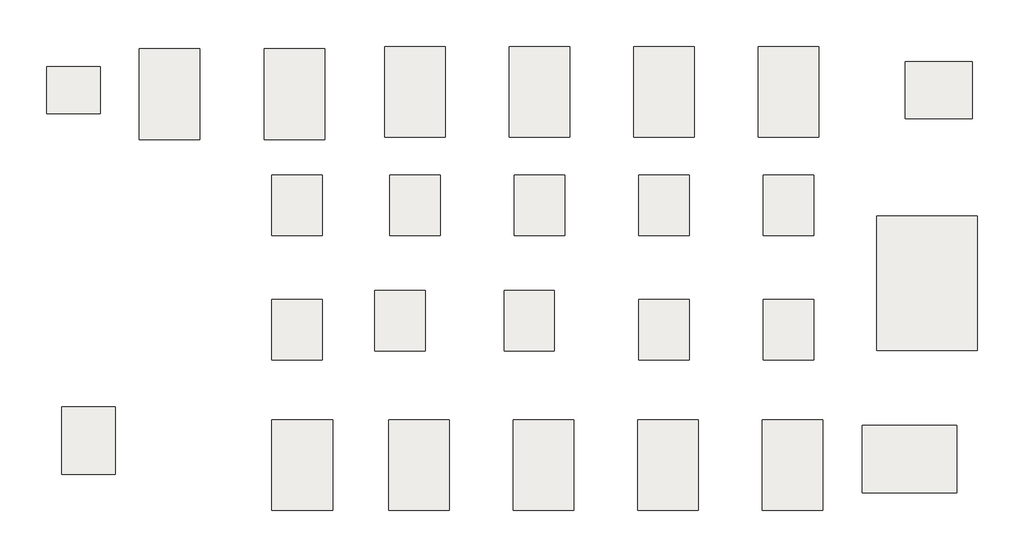
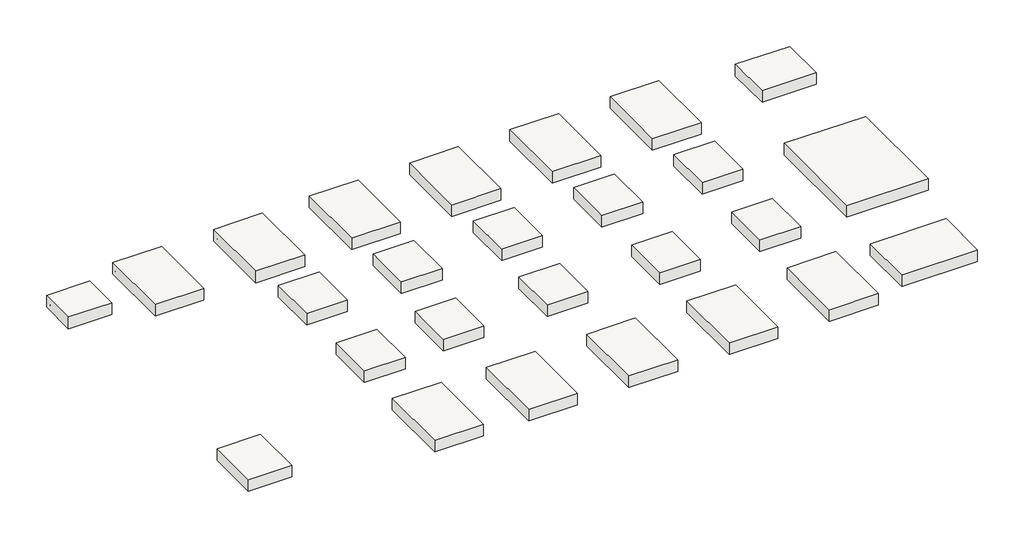
# One storey, part 1 of 2: 26 slabs.
"""IFC4 building model written with IfcOpenShell, lengths in millimetres."""

from ifc_helpers import new_model, si_unit, origin, place, context, project, spatial, transform, mapped, element, save
from components import m_footing_rectangular_1500_x_1800_x_450mm_b88d8e73, m_footing_rectangular_1600_x_1400_x_450mm_70e385b2, m_footing_rectangular_1600_x_2000_x_450mm_9aacb398, m_footing_rectangular_1800_x_2700_x_450mm_20c57781, m_footing_rectangular_2000_x_1700_x_450mm_1621679d, m_footing_rectangular_2800_x_2000_x_450mm_3d0566a5, m_footing_rectangular_3000_x_4000_x_450mm_fa7846ad

model = new_model("IFC4")

# Units and contexts
model_context = context("Model", 3, world=origin())
ifc_project = project(units=[si_unit("LENGTHUNIT", "METRE", prefix="MILLI")], contexts=[model_context])

# Site, building, storey
site = spatial("IfcSite", under=ifc_project)
building = spatial("IfcBuilding", under=site)
storey = spatial("IfcBuildingStorey", under=building, Elevation=-2133.6)

# Slabs
placement = place(None, origin())
m_footing_rectangular_1500_x_1800_x_450mm_shape = m_footing_rectangular_1500_x_1800_x_450mm_b88d8e73(model_context)
element("IfcSlab", 1, ObjectType="M_Footing-Rectangular : 1500 x 1800 x 450mm", at=placement, inside=storey, context=model_context, shape_type="MappedRepresentation", body=[
    mapped(m_footing_rectangular_1500_x_1800_x_450mm_shape, transform((-8871.6002151, 1284.1968026, -2133.6), x_axis=(1.0, 0.0, 0.0), y_axis=(0.0, 1.0, 0.0), z_axis=(0.0, 0.0, 1.0))),
])
element("IfcSlab", 2, ObjectType="M_Footing-Rectangular : 1500 x 1800 x 450mm", at=placement, inside=storey, context=model_context, shape_type="MappedRepresentation", body=[
    mapped(m_footing_rectangular_1500_x_1800_x_450mm_shape, transform((-5370.5486955, 1285.6388796, -2133.6), x_axis=(1.0, 0.0, 0.0), y_axis=(0.0, 1.0, 0.0), z_axis=(0.0, 0.0, 1.0))),
])
element("IfcSlab", 3, ObjectType="M_Footing-Rectangular : 1500 x 1800 x 450mm", at=placement, inside=storey, context=model_context, shape_type="MappedRepresentation", body=[
    mapped(m_footing_rectangular_1500_x_1800_x_450mm_shape, transform((2029.4513045, 1285.6388796, -2133.6), x_axis=(1.0, 0.0, 0.0), y_axis=(0.0, 1.0, 0.0), z_axis=(0.0, 0.0, 1.0))),
])
element("IfcSlab", 4, ObjectType="M_Footing-Rectangular : 1500 x 1800 x 450mm", at=placement, inside=storey, context=model_context, shape_type="MappedRepresentation", body=[
    mapped(m_footing_rectangular_1500_x_1800_x_450mm_shape, transform((5729.4513045, 1285.6388796, -2133.6), x_axis=(1.0, 0.0, 0.0), y_axis=(0.0, 1.0, 0.0), z_axis=(0.0, 0.0, 1.0))),
])
element("IfcSlab", 5, ObjectType="M_Footing-Rectangular : 1500 x 1800 x 450mm", at=placement, inside=storey, context=model_context, shape_type="MappedRepresentation", body=[
    mapped(m_footing_rectangular_1500_x_1800_x_450mm_shape, transform((-8870.5486955, -2415.8031974, -2133.6), x_axis=(1.0, 0.0, 0.0), y_axis=(0.0, 1.0, 0.0), z_axis=(0.0, 0.0, 1.0))),
])
element("IfcSlab", 6, ObjectType="M_Footing-Rectangular : 1500 x 1800 x 450mm", at=placement, inside=storey, context=model_context, shape_type="MappedRepresentation", body=[
    mapped(m_footing_rectangular_1500_x_1800_x_450mm_shape, transform((-5810.4090662, -2148.9247482, -2133.6), x_axis=(1.0, 0.0, 0.0), y_axis=(0.0, 1.0, 0.0), z_axis=(0.0, 0.0, 1.0))),
])
element("IfcSlab", 7, ObjectType="M_Footing-Rectangular : 1500 x 1800 x 450mm", at=placement, inside=storey, context=model_context, shape_type="MappedRepresentation", body=[
    mapped(m_footing_rectangular_1500_x_1800_x_450mm_shape, transform((-1974.31456, -2148.9247482, -2133.6), x_axis=(1.0, 0.0, 0.0), y_axis=(0.0, 1.0, 0.0), z_axis=(0.0, 0.0, 1.0))),
])
element("IfcSlab", 8, ObjectType="M_Footing-Rectangular : 1500 x 1800 x 450mm", at=placement, inside=storey, context=model_context, shape_type="MappedRepresentation", body=[
    mapped(m_footing_rectangular_1500_x_1800_x_450mm_shape, transform((2029.4513045, -2415.8031974, -2133.6), x_axis=(1.0, 0.0, 0.0), y_axis=(0.0, 1.0, 0.0), z_axis=(0.0, 0.0, 1.0))),
])
element("IfcSlab", 9, ObjectType="M_Footing-Rectangular : 1500 x 1800 x 450mm", at=placement, inside=storey, context=model_context, shape_type="MappedRepresentation", body=[
    mapped(m_footing_rectangular_1500_x_1800_x_450mm_shape, transform((5729.4513045, -2415.8031974, -2133.6), x_axis=(1.0, 0.0, 0.0), y_axis=(0.0, 1.0, 0.0), z_axis=(0.0, 0.0, 1.0))),
])
element("IfcSlab", 10, ObjectType="M_Footing-Rectangular : 1500 x 1800 x 450mm", at=placement, inside=storey, context=model_context, shape_type="MappedRepresentation", body=[
    mapped(m_footing_rectangular_1500_x_1800_x_450mm_shape, transform((-1670.5486955, 1285.6388796, -2133.6), x_axis=(1.0, 0.0, 0.0), y_axis=(0.0, 1.0, 0.0), z_axis=(0.0, 0.0, 1.0))),
])
m_footing_rectangular_1600_x_1400_x_450mm_shape = m_footing_rectangular_1600_x_1400_x_450mm_70e385b2(model_context)
element("IfcSlab", 11, ObjectType="M_Footing-Rectangular : 1600 x 1400 x 450mm", at=placement, inside=storey, context=model_context, shape_type="MappedRepresentation", body=[
    mapped(m_footing_rectangular_1600_x_1400_x_450mm_shape, transform((-15520.5877753, 4707.7547256, -2133.6), x_axis=(1.0, 0.0, 0.0), y_axis=(0.0, 1.0, 0.0), z_axis=(0.0, 0.0, 1.0))),
])
m_footing_rectangular_1600_x_2000_x_450mm_shape = m_footing_rectangular_1600_x_2000_x_450mm_9aacb398(model_context)
element("IfcSlab", 12, ObjectType="M_Footing-Rectangular : 1600 x 2000 x 450mm", at=placement, inside=storey, context=model_context, shape_type="MappedRepresentation", body=[
    mapped(m_footing_rectangular_1600_x_2000_x_450mm_shape, transform((-15072.8289366, -5717.2452744, -2133.6), x_axis=(1.0, 0.0, 0.0), y_axis=(0.0, 1.0, 0.0), z_axis=(0.0, 0.0, 1.0))),
])
m_footing_rectangular_1800_x_2700_x_450mm_shape = m_footing_rectangular_1800_x_2700_x_450mm_20c57781(model_context)
element("IfcSlab", 13, ObjectType="M_Footing-Rectangular : 1800 x 2700 x 450mm", at=placement, inside=storey, context=model_context, shape_type="MappedRepresentation", body=[
    mapped(m_footing_rectangular_1800_x_2700_x_450mm_shape, transform((-12666.802732, 4582.7547256, -2133.6), x_axis=(1.0, 0.0, 0.0), y_axis=(0.0, 1.0, 0.0), z_axis=(0.0, 0.0, 1.0))),
])
element("IfcSlab", 14, ObjectType="M_Footing-Rectangular : 1800 x 2700 x 450mm", at=placement, inside=storey, context=model_context, shape_type="MappedRepresentation", body=[
    mapped(m_footing_rectangular_1800_x_2700_x_450mm_shape, transform((-8950.302732, 4582.7547256, -2133.6), x_axis=(1.0, 0.0, 0.0), y_axis=(0.0, 1.0, 0.0), z_axis=(0.0, 0.0, 1.0))),
])
element("IfcSlab", 15, ObjectType="M_Footing-Rectangular : 1800 x 2700 x 450mm", at=placement, inside=storey, context=model_context, shape_type="MappedRepresentation", body=[
    mapped(m_footing_rectangular_1800_x_2700_x_450mm_shape, transform((-5375.302732, 4654.6486596, -2133.6), x_axis=(1.0, 0.0, 0.0), y_axis=(0.0, 1.0, 0.0), z_axis=(0.0, 0.0, 1.0))),
])
element("IfcSlab", 16, ObjectType="M_Footing-Rectangular : 1800 x 2700 x 450mm", at=placement, inside=storey, context=model_context, shape_type="MappedRepresentation", body=[
    mapped(m_footing_rectangular_1800_x_2700_x_450mm_shape, transform((-1675.302732, 4654.6486596, -2133.6), x_axis=(1.0, 0.0, 0.0), y_axis=(0.0, 1.0, 0.0), z_axis=(0.0, 0.0, 1.0))),
])
element("IfcSlab", 17, ObjectType="M_Footing-Rectangular : 1800 x 2700 x 450mm", at=placement, inside=storey, context=model_context, shape_type="MappedRepresentation", body=[
    mapped(m_footing_rectangular_1800_x_2700_x_450mm_shape, transform((2024.697268, 4654.6486596, -2133.6), x_axis=(1.0, 0.0, 0.0), y_axis=(0.0, 1.0, 0.0), z_axis=(0.0, 0.0, 1.0))),
])
element("IfcSlab", 18, ObjectType="M_Footing-Rectangular : 1800 x 2700 x 450mm", at=placement, inside=storey, context=model_context, shape_type="MappedRepresentation", body=[
    mapped(m_footing_rectangular_1800_x_2700_x_450mm_shape, transform((5724.697268, 4654.6486596, -2133.6), x_axis=(1.0, 0.0, 0.0), y_axis=(0.0, 1.0, 0.0), z_axis=(0.0, 0.0, 1.0))),
])
element("IfcSlab", 19, ObjectType="M_Footing-Rectangular : 1800 x 2700 x 450mm", at=placement, inside=storey, context=model_context, shape_type="MappedRepresentation", body=[
    mapped(m_footing_rectangular_1800_x_2700_x_450mm_shape, transform((-8720.5486955, -6446.5229254, -2133.6), x_axis=(1.0, 0.0, 0.0), y_axis=(0.0, 1.0, 0.0), z_axis=(0.0, 0.0, 1.0))),
])
element("IfcSlab", 20, ObjectType="M_Footing-Rectangular : 1800 x 2700 x 450mm", at=placement, inside=storey, context=model_context, shape_type="MappedRepresentation", body=[
    mapped(m_footing_rectangular_1800_x_2700_x_450mm_shape, transform((-5250.302732, -6446.5229254, -2133.6), x_axis=(1.0, 0.0, 0.0), y_axis=(0.0, 1.0, 0.0), z_axis=(0.0, 0.0, 1.0))),
])
element("IfcSlab", 21, ObjectType="M_Footing-Rectangular : 1800 x 2700 x 450mm", at=placement, inside=storey, context=model_context, shape_type="MappedRepresentation", body=[
    mapped(m_footing_rectangular_1800_x_2700_x_450mm_shape, transform((-1550.302732, -6446.5229254, -2133.6), x_axis=(1.0, 0.0, 0.0), y_axis=(0.0, 1.0, 0.0), z_axis=(0.0, 0.0, 1.0))),
])
element("IfcSlab", 22, ObjectType="M_Footing-Rectangular : 1800 x 2700 x 450mm", at=placement, inside=storey, context=model_context, shape_type="MappedRepresentation", body=[
    mapped(m_footing_rectangular_1800_x_2700_x_450mm_shape, transform((2149.697268, -6446.5229254, -2133.6), x_axis=(1.0, 0.0, 0.0), y_axis=(0.0, 1.0, 0.0), z_axis=(0.0, 0.0, 1.0))),
])
element("IfcSlab", 23, ObjectType="M_Footing-Rectangular : 1800 x 2700 x 450mm", at=placement, inside=storey, context=model_context, shape_type="MappedRepresentation", body=[
    mapped(m_footing_rectangular_1800_x_2700_x_450mm_shape, transform((5849.697268, -6446.5229254, -2133.6), x_axis=(1.0, 0.0, 0.0), y_axis=(0.0, 1.0, 0.0), z_axis=(0.0, 0.0, 1.0))),
])
m_footing_rectangular_2000_x_1700_x_450mm_shape = m_footing_rectangular_2000_x_1700_x_450mm_1621679d(model_context)
element("IfcSlab", 24, ObjectType="M_Footing-Rectangular : 2000 x 1700 x 450mm", at=placement, inside=storey, context=model_context, shape_type="MappedRepresentation", body=[
    mapped(m_footing_rectangular_2000_x_1700_x_450mm_shape, transform((10195.9122247, 4707.7547256, -2133.6), x_axis=(1.0, 0.0, 0.0), y_axis=(0.0, 1.0, 0.0), z_axis=(0.0, 0.0, 1.0))),
])
m_footing_rectangular_2800_x_2000_x_450mm_shape = m_footing_rectangular_2800_x_2000_x_450mm_3d0566a5(model_context)
element("IfcSlab", 25, ObjectType="M_Footing-Rectangular : 2800 x 2000 x 450mm", at=placement, inside=storey, context=model_context, shape_type="MappedRepresentation", body=[
    mapped(m_footing_rectangular_2800_x_2000_x_450mm_shape, transform((9325.9122247, -6266.2452744, -2133.6), x_axis=(1.0, 0.0, 0.0), y_axis=(0.0, 1.0, 0.0), z_axis=(0.0, 0.0, 1.0))),
])
m_footing_rectangular_3000_x_4000_x_450mm_shape = m_footing_rectangular_3000_x_4000_x_450mm_fa7846ad(model_context)
element("IfcSlab", 26, ObjectType="M_Footing-Rectangular : 3000 x 4000 x 450mm", at=placement, inside=storey, context=model_context, shape_type="MappedRepresentation", body=[
    mapped(m_footing_rectangular_3000_x_4000_x_450mm_shape, transform((9845.9122247, -1034.7452744, -2133.6), x_axis=(1.0, 0.0, 0.0), y_axis=(0.0, 1.0, 0.0), z_axis=(0.0, 0.0, 1.0))),
])

save(model, "model.ifc")

# Revit data of these elements
# Type "M_Footing-Rectangular : 1500 x 1800 x 450mm"
#   Width = 4' - 11.05512"
#   Length = 5' - 10.86614"
#   Foundation Thickness = 1' - 5.71654"
#   Structural Material [instance default] = Concrete, Cast-in-Place gray
#   Assembly Code = ""
# Type "M_Footing-Rectangular : 1600 x 1400 x 450mm"
#   Width = 5' - 2.99213"
#   Length = 4' - 7.11811"
#   Foundation Thickness = 1' - 5.71654"
#   Structural Material [instance default] = Concrete, Cast-in-Place gray
#   Assembly Code = ""
# Type "M_Footing-Rectangular : 1600 x 2000 x 450mm"
#   Width = 5' - 2.99213"
#   Length = 6' - 6.74016"
#   Foundation Thickness = 1' - 5.71654"
#   Structural Material [instance default] = Concrete, Cast-in-Place gray
#   Assembly Code = ""
# Type "M_Footing-Rectangular : 1800 x 2700 x 450mm"
#   Width = 5' - 10.86614"
#   Length = 8' - 10.29921"
#   Foundation Thickness = 1' - 5.71654"
#   Structural Material [instance default] = Concrete, Cast-in-Place gray
#   Assembly Code = ""
# Type "M_Footing-Rectangular : 2000 x 1700 x 450mm"
#   Width = 6' - 6.74016"
#   Length = 5' - 6.92913"
#   Foundation Thickness = 1' - 5.71654"
#   Structural Material [instance default] = Concrete, Cast-in-Place gray
#   Assembly Code = ""
# Type "M_Footing-Rectangular : 2800 x 2000 x 450mm"
#   Width = 9' - 2.23622"
#   Length = 6' - 6.74016"
#   Foundation Thickness = 1' - 5.71654"
#   Structural Material [instance default] = Concrete, Cast-in-Place gray
#   Assembly Code = ""
# Type "M_Footing-Rectangular : 3000 x 4000 x 450mm"
#   Width = 9' - 10.11024"
#   Length = 13' - 1.48031"
#   Foundation Thickness = 1' - 5.71654"
#   Structural Material [instance default] = Concrete, Cast-in-Place gray
#   Assembly Code = ""
# Elements 1, 2, 3, 4, 5, 6, 7, 8, 9, 10 (IfcSlab, "M_Footing-Rectangular : 1500 x 1800 x 450mm")
#   Structural Material = Concrete, Cast-in-Place gray
#   Phase Created = New Construction
#   Materials on its faces: "Concrete, Cast-in-Place gray"
# Element 11 (IfcSlab, "M_Footing-Rectangular : 1600 x 1400 x 450mm")
#   Structural Material = Concrete, Cast-in-Place gray
#   Phase Created = New Construction
#   Materials on its faces: "Concrete, Cast-in-Place gray"
# Element 12 (IfcSlab, "M_Footing-Rectangular : 1600 x 2000 x 450mm")
#   Structural Material = Concrete, Cast-in-Place gray
#   Phase Created = New Construction
#   Materials on its faces: "Concrete, Cast-in-Place gray"
# Elements 13, 14, 15, 16, 17, 18, 19, 20, 21, 22, 23 (IfcSlab, "M_Footing-Rectangular : 1800 x 2700 x 450mm")
#   Structural Material = Concrete, Cast-in-Place gray
#   Phase Created = New Construction
#   Materials on its faces: "Concrete, Cast-in-Place gray"
# Element 24 (IfcSlab, "M_Footing-Rectangular : 2000 x 1700 x 450mm")
#   Structural Material = Concrete, Cast-in-Place gray
#   Phase Created = New Construction
#   Materials on its faces: "Concrete, Cast-in-Place gray"
# Element 25 (IfcSlab, "M_Footing-Rectangular : 2800 x 2000 x 450mm")
#   Structural Material = Concrete, Cast-in-Place gray
#   Phase Created = New Construction
#   Materials on its faces: "Concrete, Cast-in-Place gray"
# Element 26 (IfcSlab, "M_Footing-Rectangular : 3000 x 4000 x 450mm")
#   Structural Material = Concrete, Cast-in-Place gray
#   Phase Created = New Construction
#   Materials on its faces: "Concrete, Cast-in-Place gray"
# Materials
#   "Concrete, Cast-in-Place gray": class "Concrete", colour RGB 192 192 192, transparency 0, Description = "Cast-in-place concrete", Cost = 0
